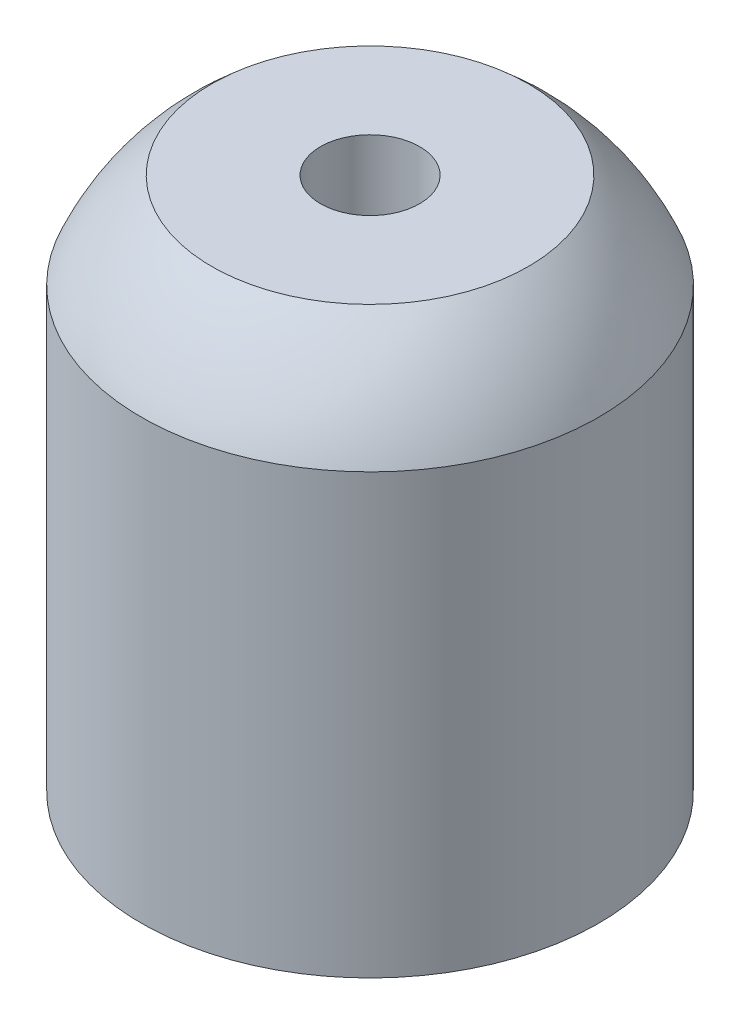
ISO-10303-21;
HEADER;
FILE_DESCRIPTION(('STEP AP214'),'2;1');
FILE_NAME('part.step','',(''),(''),'','','');
FILE_SCHEMA(('AUTOMOTIVE_DESIGN { 1 0 10303 214 1 1 1 1 }'));
ENDSEC;
DATA;
#1=APPLICATION_CONTEXT('core data for automotive mechanical design processes');
#2=APPLICATION_PROTOCOL_DEFINITION('international standard','automotive_design',2000,#1);
#3=PRODUCT_CONTEXT('',#1,'mechanical');
#4=PRODUCT('Part','Part','',(#3));
#5=PRODUCT_RELATED_PRODUCT_CATEGORY('part','',(#4));
#6=PRODUCT_DEFINITION_FORMATION('','',#4);
#7=PRODUCT_DEFINITION_CONTEXT('part definition',#1,'design');
#8=PRODUCT_DEFINITION('design','',#6,#7);
#9=PRODUCT_DEFINITION_SHAPE('','',#8);
#10=(LENGTH_UNIT() NAMED_UNIT(*) SI_UNIT(.MILLI.,.METRE.));
#11=(NAMED_UNIT(*) PLANE_ANGLE_UNIT() SI_UNIT($,.RADIAN.));
#12=(NAMED_UNIT(*) SI_UNIT($,.STERADIAN.) SOLID_ANGLE_UNIT());
#13=UNCERTAINTY_MEASURE_WITH_UNIT(LENGTH_MEASURE(1.E-05),#10,'distance_accuracy_value','');
#14=(GEOMETRIC_REPRESENTATION_CONTEXT(3) GLOBAL_UNCERTAINTY_ASSIGNED_CONTEXT((#13)) GLOBAL_UNIT_ASSIGNED_CONTEXT((#10,
#11,#12)) REPRESENTATION_CONTEXT('',''));
#15=CARTESIAN_POINT('',(0.,0.,0.));
#16=DIRECTION('',(0.,0.,1.));
#17=DIRECTION('',(1.,0.,0.));
#18=AXIS2_PLACEMENT_3D('',#15,#16,#17);
#19=CARTESIAN_POINT('',(0.,18.,0.));
#20=DIRECTION('',(0.,0.,1.));
#21=DIRECTION('',(1.,0.,0.));
#22=AXIS2_PLACEMENT_3D('',#19,#20,#21);
#23=SPHERICAL_SURFACE('',#22,13.);
#24=CARTESIAN_POINT('',(0.,18.,0.));
#25=DIRECTION('',(0.,-1.,0.));
#26=DIRECTION('',(0.,0.,-1.));
#27=AXIS2_PLACEMENT_3D('',#24,#25,#26);
#28=SPHERICAL_SURFACE('',#27,13.);
#29=CARTESIAN_POINT('',(0.,28.,0.));
#30=DIRECTION('',(0.,-1.,0.));
#31=DIRECTION('',(0.,0.,-1.));
#32=AXIS2_PLACEMENT_3D('',#29,#30,#31);
#33=CIRCLE('',#32,8.30662386291807);
#34=CARTESIAN_POINT('',(0.,28.,-8.30662386291807));
#35=VERTEX_POINT('',#34);
#36=EDGE_CURVE('E50',#35,#35,#33,.T.);
#37=ORIENTED_EDGE('',*,*,#36,.T.);
#38=EDGE_LOOP('',(#37));
#39=FACE_BOUND('',#38,.T.);
#40=CARTESIAN_POINT('',(0.,23.,0.));
#41=DIRECTION('',(0.,-1.,0.));
#42=DIRECTION('',(0.,0.,-1.));
#43=AXIS2_PLACEMENT_3D('',#40,#41,#42);
#44=CIRCLE('',#43,12.);
#45=CARTESIAN_POINT('',(0.,23.,-12.));
#46=VERTEX_POINT('',#45);
#47=EDGE_CURVE('E11',#46,#46,#44,.T.);
#48=ORIENTED_EDGE('',*,*,#47,.F.);
#49=EDGE_LOOP('',(#48));
#50=FACE_BOUND('',#49,.T.);
#51=ADVANCED_FACE('F42',(#39,#50),#28,.T.);
#52=CARTESIAN_POINT('',(0.,0.,0.));
#53=DIRECTION('',(0.,-1.,0.));
#54=DIRECTION('',(0.,0.,-1.));
#55=AXIS2_PLACEMENT_3D('',#52,#53,#54);
#56=CYLINDRICAL_SURFACE('',#55,12.);
#57=CARTESIAN_POINT('',(0.,0.,0.));
#58=DIRECTION('',(0.,-1.,0.));
#59=DIRECTION('',(0.,0.,-1.));
#60=AXIS2_PLACEMENT_3D('',#57,#58,#59);
#61=CIRCLE('',#60,12.);
#62=CARTESIAN_POINT('',(0.,0.,-12.));
#63=VERTEX_POINT('',#62);
#64=EDGE_CURVE('E51',#63,#63,#61,.T.);
#65=ORIENTED_EDGE('',*,*,#64,.F.);
#66=EDGE_LOOP('',(#65));
#67=FACE_BOUND('',#66,.T.);
#68=ORIENTED_EDGE('',*,*,#47,.T.);
#69=EDGE_LOOP('',(#68));
#70=FACE_BOUND('',#69,.T.);
#71=ADVANCED_FACE('F85',(#67,#70),#56,.T.);
#72=CARTESIAN_POINT('',(0.,0.,0.));
#73=DIRECTION('',(0.,1.,0.));
#74=DIRECTION('',(0.,0.,1.));
#75=AXIS2_PLACEMENT_3D('',#72,#73,#74);
#76=PLANE('',#75);
#77=ORIENTED_EDGE('',*,*,#64,.T.);
#78=EDGE_LOOP('',(#77));
#79=FACE_BOUND('',#78,.T.);
#80=ADVANCED_FACE('F75',(#79),#76,.F.);
#81=CARTESIAN_POINT('',(0.,28.,0.));
#82=DIRECTION('',(0.,-1.,0.));
#83=DIRECTION('',(0.,0.,-1.));
#84=AXIS2_PLACEMENT_3D('',#81,#82,#83);
#85=PLANE('',#84);
#86=CARTESIAN_POINT('',(0.,28.,0.));
#87=DIRECTION('',(0.,1.,0.));
#88=DIRECTION('',(0.,0.,1.));
#89=AXIS2_PLACEMENT_3D('',#86,#87,#88);
#90=CIRCLE('',#89,2.6);
#91=CARTESIAN_POINT('',(0.,28.,2.6));
#92=VERTEX_POINT('',#91);
#93=EDGE_CURVE('E60',#92,#92,#90,.T.);
#94=ORIENTED_EDGE('',*,*,#93,.F.);
#95=EDGE_LOOP('',(#94));
#96=FACE_BOUND('',#95,.T.);
#97=ORIENTED_EDGE('',*,*,#36,.F.);
#98=EDGE_LOOP('',(#97));
#99=FACE_BOUND('',#98,.T.);
#100=ADVANCED_FACE('F70',(#96,#99),#85,.F.);
#101=CARTESIAN_POINT('',(0.,18.,0.));
#102=DIRECTION('',(0.,1.,0.));
#103=DIRECTION('',(0.,0.,1.));
#104=AXIS2_PLACEMENT_3D('',#101,#102,#103);
#105=CYLINDRICAL_SURFACE('',#104,2.6);
#106=CARTESIAN_POINT('',(0.,18.,0.));
#107=DIRECTION('',(0.,1.,0.));
#108=DIRECTION('',(0.,0.,1.));
#109=AXIS2_PLACEMENT_3D('',#106,#107,#108);
#110=CIRCLE('',#109,2.6);
#111=CARTESIAN_POINT('',(0.,18.,2.6));
#112=VERTEX_POINT('',#111);
#113=EDGE_CURVE('E58',#112,#112,#110,.T.);
#114=ORIENTED_EDGE('',*,*,#113,.F.);
#115=EDGE_LOOP('',(#114));
#116=FACE_BOUND('',#115,.T.);
#117=ORIENTED_EDGE('',*,*,#93,.T.);
#118=EDGE_LOOP('',(#117));
#119=FACE_BOUND('',#118,.T.);
#120=ADVANCED_FACE('F72',(#116,#119),#105,.F.);
#121=CARTESIAN_POINT('',(0.,18.,0.));
#122=DIRECTION('',(0.,1.,0.));
#123=DIRECTION('',(0.,0.,1.));
#124=AXIS2_PLACEMENT_3D('',#121,#122,#123);
#125=PLANE('',#124);
#126=ORIENTED_EDGE('',*,*,#113,.T.);
#127=EDGE_LOOP('',(#126));
#128=FACE_BOUND('',#127,.T.);
#129=ADVANCED_FACE('F79',(#128),#125,.T.);
#130=CLOSED_SHELL('',(#51,#71,#80,#100,#120,#129));
#131=MANIFOLD_SOLID_BREP('B2',#130);
#132=ADVANCED_BREP_SHAPE_REPRESENTATION('',(#18,#131),#14);
#133=SHAPE_DEFINITION_REPRESENTATION(#9,#132);
ENDSEC;
END-ISO-10303-21;
